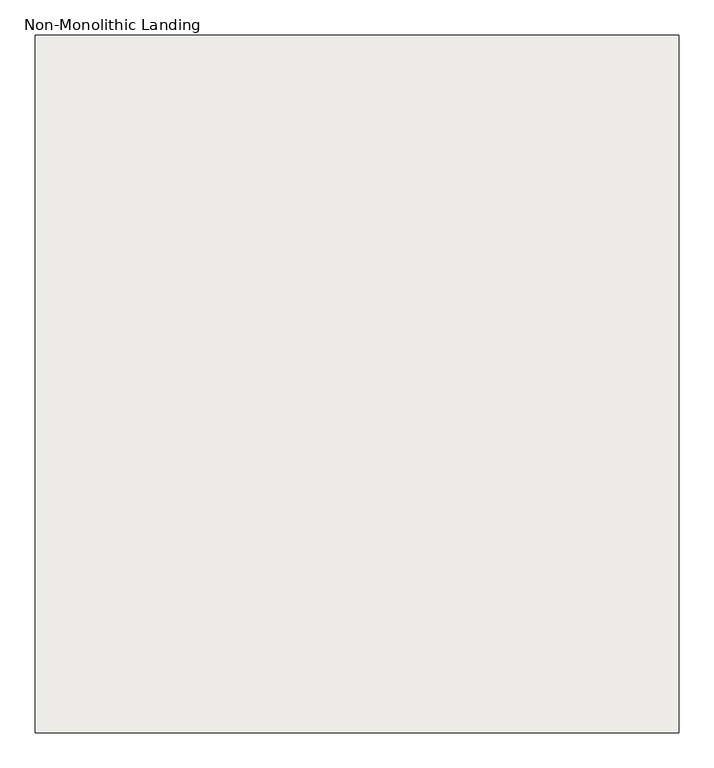
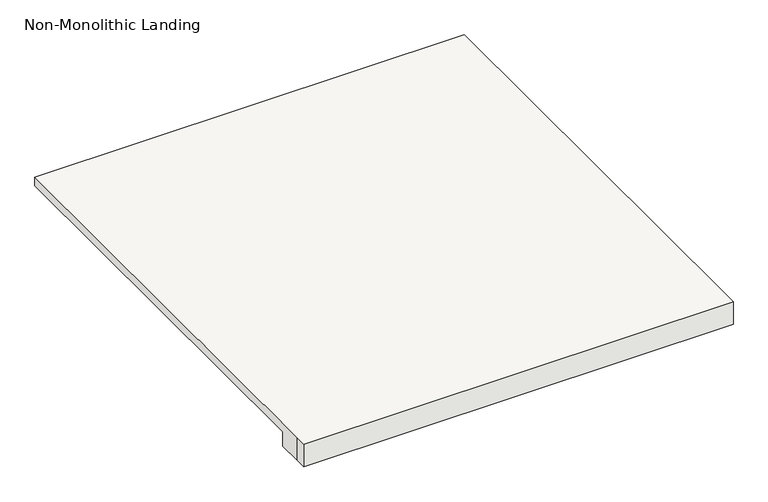
"""IFC4 building model written with IfcOpenShell, lengths in millimetres: slab geometry, Non-Monolithic Landing."""

from ifc_helpers import new_model, si_unit, origin, place, context, project, spatial, faceted_brep, source, transform, mapped, element, save


def non_monolithic_landing_e7e36702(model_context):
    return source(origin(), model_context, "Body", "Brep", [
        faceted_brep([(-803.1608498, 4479.7115866, 4214.2833333), (-777.7608498, 4479.7115866, 4188.8833333), (-777.7608498, 3565.3115866, 4188.8833333), (-803.1608498, 3565.3115866, 4214.2833333), (-803.1608498, 3514.5115866, 4233.3333333), (-803.1608498, 3489.1115866, 4233.3333333), (111.2391502, 3489.1115866, 4233.3333333), (111.2391502, 3514.5115866, 4233.3333333), (111.2391502, 4479.7115866, 4233.3333333), (-803.1608498, 4479.7115866, 4233.3333333), (-777.7608498, 3565.3115866, 4182.5333333), (-777.7608498, 4479.7115866, 4182.5333333), (111.2391502, 4479.7115866, 4182.5333333), (111.2391502, 3514.5115866, 4182.5333333), (111.2391502, 3489.1115866, 4182.5333333), (-803.1608498, 3489.1115866, 4182.5333333), (-803.1608498, 3514.5115866, 4182.5333333), (-803.1608498, 3565.3115866, 4182.5333333)], [[[0, 1, 2, 3]], [[4, 5, 6, 7, 8, 9]], [[10, 11, 12, 13, 14, 15, 16, 17]], [[11, 10, 2, 1]], [[10, 17, 3, 2]], [[4, 9, 0, 3, 17, 16]], [[5, 4, 16, 15]], [[6, 5, 15, 14]], [[7, 6, 14, 13]], [[8, 7, 13, 12]], [[9, 8, 12, 11, 1, 0]]]),
    ])


if __name__ == "__main__":
    model = new_model("IFC4")
    model_context = context("Model", 3, world=origin())
    ifc_project = project(units=[si_unit("LENGTHUNIT", "METRE", prefix="MILLI")], contexts=[model_context])
    site = spatial("IfcSite", under=ifc_project)
    building = spatial("IfcBuilding", under=site)
    placement = place(None, origin())
    non_monolithic_landing_shape = non_monolithic_landing_e7e36702(model_context)
    element("IfcSlab", 1, ObjectType="Non-Monolithic Landing", at=placement, inside=building, context=model_context, shape_type="MappedRepresentation", body=[
        mapped(non_monolithic_landing_shape, transform((0.0, 0.0, 0.0), x_axis=(1.0, 0.0, 0.0), y_axis=(0.0, 1.0, 0.0), z_axis=(0.0, 0.0, 1.0))),
    ])
    save(model, "model.ifc")
